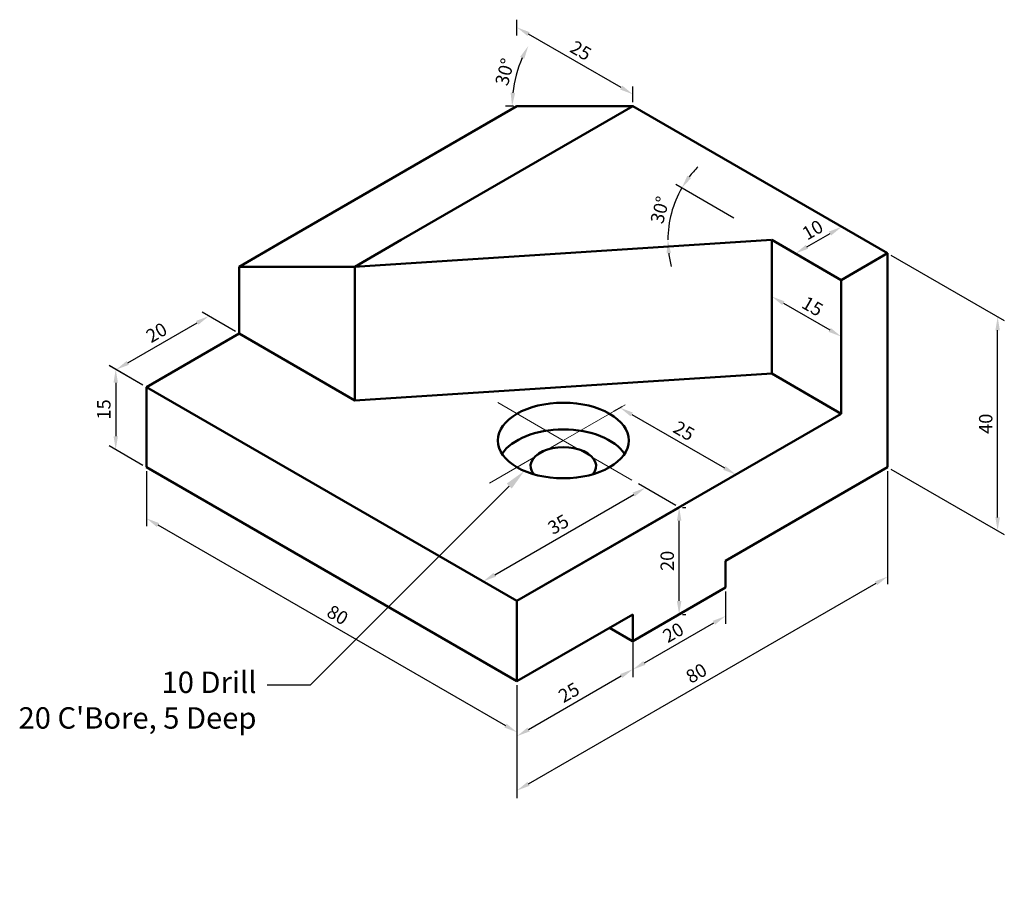
# Model space of a CAD drawing. Units: millimetres. Extents: x 2441 to 2625, y 4324 to 4485.
import ezdxf
from ezdxf import colors
from ezdxf.entities.mleader import LeaderData, LeaderLine
from ezdxf.math import Vec2, Vec3

# ---------------------------------------------------------------- set-up
doc = ezdxf.new("R2010")
doc.units = ezdxf.units.MM
doc.linetypes.add('CENTER', pattern=[50.8, 31.75, -6.35, 6.35, -6.35])
for name, color, linetype, lineweight in [('M-CNTR', 4, 'CENTER', 18), ('M-DIMS', 2, 'Continuous', 25), ('M-OUTL', 7, 'Continuous', 50), ('M-TEXT', 7, 'Continuous', 25)]:
    doc.layers.add(name, color=color, linetype=linetype, lineweight=lineweight)
doc.styles.get("Standard").update_dxf_attribs({"font": 'arial.ttf'})
doc.dimstyles.new('ISO-25', dxfattribs={"dimtxt": 2.5, "dimasz": 2.5, "dimexe": 1.25, "dimexo": 0.625, "dimtad": 1, "dimtxsty": 'Standard', "dimcen": 2.5, "dimadec": 0, "dimazin": 0, "dimtfac": 1, "dimtmove": 0, "dimatfit": 3, "dimfxl": 1, "dimarcsym": 0})

# ---------------------------------------------------------------- blocks, each defined once
blk = doc.blocks.new('*D1')
at = {"layer": 'Defpoints', "color": 0, "transparency": 16777216}
for p in [(2594.92, 4446.26), (2603.5, 4441.3), (2594.84, 4436.3)]:
    blk.add_point(p, dxfattribs=at)
at = {"layer": 'M-DIMS', "color": 0, "lineweight": -2, "transparency": 16777216}
for p, q in [((2602.88, 4441.66), (2593.67, 4446.98)), ((2588.42, 4442.51), (2592.75, 4445.01)), ((2594.22, 4436.66), (2585.01, 4441.98))]:
    blk.add_line(p, q, dxfattribs=at)
at = {"layer": 'M-DIMS', "color": 0, "transparency": 16777216}
for points in [[(2592.54, 4445.37), (2592.96, 4444.65), (2594.92, 4446.26)], [(2588.21, 4442.87), (2588.63, 4442.15), (2586.26, 4441.26)]]:
    blk.add_solid(points, dxfattribs=at)
at = {"layer": 'M-DIMS', "color": 0, "transparency": 16777216, "insert": (2589.64, 4445.41), "char_height": 2.5, "attachment_point": 5, "rotation": 30}
blk.add_mtext('10', dxfattribs=at)
blk = doc.blocks.new('*D2')
at = {"layer": 'Defpoints', "color": 0, "transparency": 16777216}
for p in [(2534.22, 4483.54), (2534.22, 4481.3), (2555.87, 4468.8)]:
    blk.add_point(p, dxfattribs=at)
at = {"layer": 'M-DIMS', "color": 0, "lineweight": -2, "transparency": 16777216}
for p, q in [((2534.22, 4482.03), (2534.22, 4484.98)), ((2553.7, 4472.29), (2536.38, 4482.29)), ((2555.87, 4469.53), (2555.87, 4472.48))]:
    blk.add_line(p, q, dxfattribs=at)
at = {"layer": 'M-DIMS', "color": 0, "transparency": 16777216}
for points in [[(2536.59, 4482.65), (2536.18, 4481.93), (2534.22, 4483.54)], [(2553.91, 4472.65), (2553.5, 4471.93), (2555.87, 4471.04)]]:
    blk.add_solid(points, dxfattribs=at)
at = {"layer": 'M-DIMS', "color": 0, "transparency": 16777216, "insert": (2545.99, 4478.93), "char_height": 2.5, "attachment_point": 5, "rotation": 330}
blk.add_mtext('25', dxfattribs=at)
blk = doc.blocks.new('*D3')
at = {"layer": 'Defpoints', "color": 0, "transparency": 16777216}
for p in [(2534.22, 4481.3), (2534.67, 4476.52), (2534.22, 4468.8), (2555.87, 4468.8), (2555.87, 4468.8)]:
    blk.add_point(p, dxfattribs=at)
at = {"layer": 'M-DIMS', "color": 0, "lineweight": -2, "transparency": 16777216}
blk.add_line((2533.59, 4468.8), (2532.06, 4468.8), dxfattribs=at)
blk.add_arc((2555.87, 4468.8), 22.56, 156.3532, 173.6468, dxfattribs=at)
at = {"layer": 'M-DIMS', "color": 0, "transparency": 16777216}
for points in [[(2534.83, 4478.04), (2535.58, 4477.66), (2536.33, 4480.08)], [(2533.87, 4471.28), (2533.03, 4471.32), (2533.31, 4468.8)]]:
    blk.add_solid(points, dxfattribs=at)
at = {"layer": 'M-DIMS', "color": 0, "transparency": 16777216, "insert": (2532.24, 4475.13), "char_height": 2.5, "attachment_point": 5, "rotation": 75}
blk.add_mtext('30°', dxfattribs=at)
blk = doc.blocks.new('*D4')
at = {"layer": 'Defpoints', "color": 0, "transparency": 16777216}
for p in [(2603.5, 4441.3), (2624.06, 4429.43), (2603.5, 4401.3)]:
    blk.add_point(p, dxfattribs=at)
at = {"layer": 'M-DIMS', "color": 0, "lineweight": -2, "transparency": 16777216}
for p, q in [((2604.13, 4440.94), (2625.31, 4428.71)), ((2624.06, 4391.93), (2624.06, 4426.93)), ((2604.13, 4400.94), (2625.31, 4388.71))]:
    blk.add_line(p, q, dxfattribs=at)
at = {"layer": 'M-DIMS', "color": 0, "transparency": 16777216}
for points in [[(2623.65, 4426.93), (2624.48, 4426.93), (2624.06, 4429.43)], [(2623.65, 4391.93), (2624.48, 4391.93), (2624.06, 4389.43)]]:
    blk.add_solid(points, dxfattribs=at)
at = {"layer": 'M-DIMS', "color": 0, "transparency": 16777216, "insert": (2622.16, 4409.43), "char_height": 2.5, "attachment_point": 5, "rotation": 90}
blk.add_mtext('40', dxfattribs=at)
blk = doc.blocks.new('*D5')
at = {"layer": 'Defpoints', "color": 0, "transparency": 16777216}
for p in [(2476.61, 4429.56), (2482.26, 4426.3), (2464.94, 4416.3)]:
    blk.add_point(p, dxfattribs=at)
at = {"layer": 'M-DIMS', "color": 0, "lineweight": -2, "transparency": 16777216}
for p, q in [((2481.63, 4426.66), (2475.36, 4430.28)), ((2461.46, 4420.81), (2474.45, 4428.31)), ((2464.31, 4416.66), (2458.04, 4420.28))]:
    blk.add_line(p, q, dxfattribs=at)
at = {"layer": 'M-DIMS', "color": 0, "transparency": 16777216}
for points in [[(2474.24, 4428.67), (2474.66, 4427.95), (2476.61, 4429.56)], [(2461.25, 4421.17), (2461.67, 4420.45), (2459.29, 4419.56)]]:
    blk.add_solid(points, dxfattribs=at)
at = {"layer": 'M-DIMS', "color": 0, "transparency": 16777216, "insert": (2467, 4426.21), "char_height": 2.5, "attachment_point": 5, "rotation": 30}
blk.add_mtext('20', dxfattribs=at)
blk = doc.blocks.new('*D6')
at = {"layer": 'Defpoints', "color": 0, "transparency": 16777216}
for p in [(2464.94, 4416.3), (2459.21, 4404.61), (2464.94, 4401.3)]:
    blk.add_point(p, dxfattribs=at)
at = {"layer": 'M-DIMS', "color": 0, "lineweight": -2, "transparency": 16777216}
for p, q in [((2464.31, 4416.66), (2457.96, 4420.33)), ((2459.21, 4417.11), (2459.21, 4407.11)), ((2464.31, 4401.66), (2457.96, 4405.33))]:
    blk.add_line(p, q, dxfattribs=at)
at = {"layer": 'M-DIMS', "color": 0, "transparency": 16777216}
for points in [[(2458.8, 4417.11), (2459.63, 4417.11), (2459.21, 4419.61)], [(2458.8, 4407.11), (2459.63, 4407.11), (2459.21, 4404.61)]]:
    blk.add_solid(points, dxfattribs=at)
at = {"layer": 'M-DIMS', "color": 0, "transparency": 16777216, "insert": (2457.31, 4412.11), "char_height": 2.5, "attachment_point": 5, "rotation": 90}
blk.add_mtext('15', dxfattribs=at)
blk = doc.blocks.new('*D7')
at = {"layer": 'Defpoints', "color": 0, "transparency": 16777216}
for p in [(2464.94, 4401.3), (2534.22, 4361.3), (2534.22, 4351.76)]:
    blk.add_point(p, dxfattribs=at)
at = {"layer": 'M-DIMS', "color": 0, "lineweight": -2, "transparency": 16777216}
for p, q in [((2464.94, 4400.58), (2464.94, 4390.32)), ((2467.1, 4390.51), (2532.05, 4353.01)), ((2534.22, 4360.58), (2534.22, 4350.32))]:
    blk.add_line(p, q, dxfattribs=at)
at = {"layer": 'M-DIMS', "color": 0, "transparency": 16777216}
for points in [[(2467.31, 4390.87), (2466.89, 4390.15), (2464.94, 4391.76)], [(2532.26, 4353.37), (2531.85, 4352.65), (2534.22, 4351.76)]]:
    blk.add_solid(points, dxfattribs=at)
at = {"layer": 'M-DIMS', "color": 0, "transparency": 16777216, "insert": (2500.53, 4373.41), "char_height": 2.5, "attachment_point": 5, "rotation": 330}
blk.add_mtext('80', dxfattribs=at)
blk = doc.blocks.new('*D8')
at = {"layer": 'Defpoints', "color": 0, "transparency": 16777216}
for p in [(2555.87, 4373.8), (2555.87, 4363.53), (2534.22, 4361.3)]:
    blk.add_point(p, dxfattribs=at)
at = {"layer": 'M-DIMS', "color": 0, "lineweight": -2, "transparency": 16777216}
for p, q in [((2555.87, 4373.08), (2555.87, 4362.08)), ((2536.38, 4352.28), (2553.7, 4362.28)), ((2534.22, 4360.58), (2534.22, 4349.58))]:
    blk.add_line(p, q, dxfattribs=at)
at = {"layer": 'M-DIMS', "color": 0, "transparency": 16777216}
for points in [[(2553.5, 4362.64), (2553.91, 4361.91), (2555.87, 4363.53)], [(2536.18, 4352.64), (2536.59, 4351.91), (2534.22, 4351.03)]]:
    blk.add_solid(points, dxfattribs=at)
at = {"layer": 'M-DIMS', "color": 0, "transparency": 16777216, "insert": (2544.09, 4358.92), "char_height": 2.5, "attachment_point": 5, "rotation": 30}
blk.add_mtext('25', dxfattribs=at)
blk = doc.blocks.new('*D9')
at = {"layer": 'Defpoints', "color": 0, "transparency": 16777216}
for p in [(2573.19, 4378.8), (2573.19, 4373.48), (2555.87, 4368.8)]:
    blk.add_point(p, dxfattribs=at)
at = {"layer": 'M-DIMS', "color": 0, "lineweight": -2, "transparency": 16777216}
for p, q in [((2573.19, 4378.08), (2573.19, 4372.04)), ((2558.03, 4364.73), (2571.02, 4372.23)), ((2555.87, 4368.08), (2555.87, 4362.04))]:
    blk.add_line(p, q, dxfattribs=at)
at = {"layer": 'M-DIMS', "color": 0, "transparency": 16777216}
for points in [[(2570.82, 4372.59), (2571.23, 4371.87), (2573.19, 4373.48)], [(2557.83, 4365.09), (2558.24, 4364.37), (2555.87, 4363.48)]]:
    blk.add_solid(points, dxfattribs=at)
at = {"layer": 'M-DIMS', "color": 0, "transparency": 16777216, "insert": (2563.58, 4370.13), "char_height": 2.5, "attachment_point": 5, "rotation": 30}
blk.add_mtext('20', dxfattribs=at)
blk = doc.blocks.new('*D10')
at = {"layer": 'Defpoints', "color": 0, "transparency": 16777216}
for p in [(2603.5, 4401.3), (2603.5, 4380.87), (2534.22, 4361.3)]:
    blk.add_point(p, dxfattribs=at)
at = {"layer": 'M-DIMS', "color": 0, "lineweight": -2, "transparency": 16777216}
for p, q in [((2603.5, 4400.58), (2603.5, 4379.43)), ((2536.38, 4342.12), (2601.34, 4379.62)), ((2534.22, 4360.58), (2534.22, 4339.43))]:
    blk.add_line(p, q, dxfattribs=at)
at = {"layer": 'M-DIMS', "color": 0, "transparency": 16777216}
for points in [[(2601.13, 4379.98), (2601.54, 4379.26), (2603.5, 4380.87)], [(2536.18, 4342.48), (2536.59, 4341.76), (2534.22, 4340.87)]]:
    blk.add_solid(points, dxfattribs=at)
at = {"layer": 'M-DIMS', "color": 0, "transparency": 16777216, "insert": (2567.91, 4362.52), "char_height": 2.5, "attachment_point": 5, "rotation": 30}
blk.add_mtext('80', dxfattribs=at)
blk = doc.blocks.new('*D11')
at = {"layer": 'Defpoints', "color": 0, "transparency": 16777216}
for p in [(2564.53, 4393.8), (2564.53, 4393.8), (2564.53, 4373.8)]:
    blk.add_point(p, dxfattribs=at)
at = {"layer": 'M-DIMS', "color": 0, "lineweight": -2, "transparency": 16777216}
for p, q in [((2565.15, 4393.8), (2565.78, 4393.8)), ((2564.53, 4376.3), (2564.53, 4391.3)), ((2565.15, 4373.8), (2565.78, 4373.8))]:
    blk.add_line(p, q, dxfattribs=at)
at = {"layer": 'M-DIMS', "color": 0, "transparency": 16777216}
for points in [[(2564.11, 4391.3), (2564.95, 4391.3), (2564.53, 4393.8)], [(2564.11, 4376.3), (2564.95, 4376.3), (2564.53, 4373.8)]]:
    blk.add_solid(points, dxfattribs=at)
at = {"layer": 'M-DIMS', "color": 0, "transparency": 16777216, "insert": (2562.63, 4383.8), "char_height": 2.5, "attachment_point": 5, "rotation": 90}
blk.add_mtext('20', dxfattribs=at)
blk = doc.blocks.new('*D12')
at = {"layer": 'Defpoints', "color": 0, "transparency": 16777216}
for p in [(2558.2, 4397.46), (2564.53, 4393.8), (2534.22, 4376.3)]:
    blk.add_point(p, dxfattribs=at)
at = {"layer": 'M-DIMS', "color": 0, "lineweight": -2, "transparency": 16777216}
for p, q in [((2563.9, 4394.16), (2556.95, 4398.18)), ((2530.06, 4381.21), (2556.04, 4396.21)), ((2533.59, 4376.66), (2526.64, 4380.68))]:
    blk.add_line(p, q, dxfattribs=at)
at = {"layer": 'M-DIMS', "color": 0, "transparency": 16777216}
for points in [[(2555.83, 4396.57), (2556.25, 4395.84), (2558.2, 4397.46)], [(2529.85, 4381.57), (2530.27, 4380.84), (2527.89, 4379.96)]]:
    blk.add_solid(points, dxfattribs=at)
at = {"layer": 'M-DIMS', "color": 0, "transparency": 16777216, "insert": (2542.1, 4390.35), "char_height": 2.5, "attachment_point": 5, "rotation": 30}
blk.add_mtext('35', dxfattribs=at)
blk = doc.blocks.new('*D13')
at = {"layer": 'Defpoints', "color": 0, "transparency": 16777216}
for p in [(2554.46, 4412.99), (2575.14, 4399.93), (2576.11, 4400.49)]:
    blk.add_point(p, dxfattribs=at)
at = {"layer": 'M-DIMS', "color": 0, "lineweight": -2, "transparency": 16777216}
for p, q in [((2553.83, 4412.63), (2552.24, 4411.71)), ((2555.66, 4411.18), (2572.98, 4401.18)), ((2575.48, 4400.13), (2573.89, 4399.21))]:
    blk.add_line(p, q, dxfattribs=at)
at = {"layer": 'M-DIMS', "color": 0, "transparency": 16777216}
for points in [[(2555.87, 4411.54), (2555.45, 4410.82), (2553.49, 4412.43)], [(2573.19, 4401.54), (2572.77, 4400.82), (2575.14, 4399.93)]]:
    blk.add_solid(points, dxfattribs=at)
at = {"layer": 'M-DIMS', "color": 0, "transparency": 16777216, "insert": (2565.27, 4407.83), "char_height": 2.5, "attachment_point": 5, "rotation": 330}
blk.add_mtext('25', dxfattribs=at)
blk = doc.blocks.new('*D14')
at = {"layer": 'Defpoints', "color": 0, "transparency": 16777216}
for p in [(2581.85, 4443.8), (2594.84, 4436.3), (2594.84, 4425.73)]:
    blk.add_point(p, dxfattribs=at)
at = {"layer": 'M-DIMS', "color": 0, "lineweight": -2, "transparency": 16777216}
for p, q in [((2581.85, 4443.08), (2581.85, 4431.78)), ((2594.84, 4435.58), (2594.84, 4424.28)), ((2584.02, 4431.98), (2592.68, 4426.98))]:
    blk.add_line(p, q, dxfattribs=at)
at = {"layer": 'M-DIMS', "color": 0, "transparency": 16777216}
for points in [[(2584.22, 4432.34), (2583.81, 4431.62), (2581.85, 4433.23)], [(2592.88, 4427.34), (2592.47, 4426.62), (2594.84, 4425.73)]]:
    blk.add_solid(points, dxfattribs=at)
at = {"layer": 'M-DIMS', "color": 0, "transparency": 16777216, "insert": (2589.3, 4431.12), "char_height": 2.5, "attachment_point": 5, "rotation": 330}
blk.add_mtext('15', dxfattribs=at)
blk = doc.blocks.new('*D15')
at = {"layer": 'Defpoints', "color": 0, "transparency": 16777216}
for p in [(2563.6, 4450.45), (2575.32, 4447.57), (2512.57, 4443.8), (2581.85, 4443.8), (2581.85, 4443.8)]:
    blk.add_point(p, dxfattribs=at)
at = {"layer": 'M-DIMS', "color": 0, "lineweight": -2, "transparency": 16777216}
blk.add_line((2574.78, 4447.88), (2563.94, 4454.14), dxfattribs=at)
for start, end in [(135.243, 142.6215), (150, 180), (187.3785, 194.757)]:
    blk.add_arc((2581.85, 4443.8), 19.43, start, end, dxfattribs=at)
at = {"layer": 'M-DIMS', "color": 0, "transparency": 16777216}
for points in [[(2566.76, 4455.37), (2566.07, 4455.83), (2565.03, 4453.52)], [(2562.17, 4441.28), (2563, 4441.34), (2562.42, 4443.8)]]:
    blk.add_solid(points, dxfattribs=at)
at = {"layer": 'M-DIMS', "color": 0, "transparency": 16777216, "insert": (2561.25, 4449.32), "char_height": 2.5, "attachment_point": 5, "rotation": 75}
blk.add_mtext('30°', dxfattribs=at)

msp = doc.modelspace()

# ---------------------------------------------------------------- linework, layer by layer
at = {"layer": 'M-CNTR'}
for p, q in [((2542.879, 4406.303), (2530.61, 4413.387)), ((2542.879, 4406.303), (2554.459, 4412.989)), ((2542.879, 4406.303), (2529.107, 4398.352)), ((2555.683, 4398.911), (2542.879, 4406.303))]:
    msp.add_line(p, q, dxfattribs=at)
at = {"layer": 'M-OUTL'}
for p, q in [((2534.219, 4468.803), (2490.173, 4443.373)), ((2555.869, 4468.803), (2512.568, 4443.803)), ((2555.869, 4468.803), (2534.219, 4468.803)), ((2603.501, 4441.303), (2555.869, 4468.803)), ((2490.173, 4443.373), (2482.257, 4438.803)), ((2503.868, 4438.803), (2581.81, 4443.803)), ((2512.568, 4443.803), (2503.908, 4438.803)), ((2594.841, 4436.303), (2581.85, 4443.803)), ((2594.841, 4436.303), (2581.85, 4443.803)), ((2581.85, 4443.803), (2581.85, 4418.803)), ((2603.501, 4441.303), (2594.841, 4436.303)), ((2603.501, 4401.303), (2603.501, 4441.303)), ((2482.257, 4426.303), (2482.257, 4438.803)), ((2482.257, 4438.803), (2503.908, 4438.803)), ((2503.908, 4413.803), (2503.908, 4438.803)), ((2594.841, 4436.303), (2594.841, 4411.303)), ((2464.937, 4416.303), (2482.257, 4426.303)), ((2482.257, 4426.303), (2495.248, 4418.803)), ((2482.257, 4426.303), (2503.908, 4413.803)), ((2503.908, 4413.803), (2503.908, 4422.919)), ((2581.85, 4418.803), (2503.908, 4413.803)), ((2594.841, 4411.303), (2581.85, 4418.803)), ((2534.219, 4376.303), (2464.937, 4416.303)), ((2464.937, 4416.303), (2464.937, 4401.303)), ((2534.219, 4376.303), (2594.841, 4411.303)), ((2464.937, 4401.303), (2534.219, 4361.303)), ((2573.19, 4383.803), (2603.501, 4401.303)), ((2534.219, 4376.303), (2564.53, 4393.803)), ((2573.19, 4383.803), (2573.19, 4378.803)), ((2555.869, 4368.803), (2573.19, 4378.803)), ((2534.219, 4361.303), (2534.219, 4376.303)), ((2534.219, 4361.303), (2555.869, 4373.803)), ((2534.219, 4361.303), (2555.869, 4373.803)), ((2555.869, 4373.803), (2555.869, 4368.803)), ((2555.869, 4373.803), (2555.869, 4368.803)), ((2555.829, 4368.803), (2551.499, 4371.303))]:
    msp.add_line(p, q, dxfattribs=at)
msp.add_ellipse((2542.879, 4406.303), major_axis=(-12.247, 0), ratio=0.5773503, dxfattribs=at)
for centre, major_axis, start_param, end_param in [((2542.879, 4401.303), (-12.247, 0), 3.5029598, 5.9218182), ((2542.879, 4401.519), (-6.124, 0), 2.6951189, 6.7296591)]:
    msp.add_ellipse(centre, major_axis=major_axis, ratio=0.5773503, start_param=start_param, end_param=end_param, dxfattribs=at)

# ---------------------------------------------------------------- dimensions: what is measured, and where the dimension line sits
at = {"layer": 'M-DIMS'}
for p1, p2, distance, picture, middle in [((2555.869, 4468.803), (2534.219, 4481.303), -1.934, '*D2', (2545.995, 4478.933)), ((2594.841, 4436.303), (2603.501, 4441.303), 8.583, '*D1', (2589.637, 4445.406)), ((2581.85, 4443.803), (2594.841, 4436.303), -9.158, '*D14', (2589.296, 4431.125)), ((2464.937, 4416.303), (2482.257, 4426.303), 5.643, '*D5', (2467.003, 4426.208)), ((2464.937, 4416.303), (2464.937, 4401.303), -5.725, '*D6', (2457.311, 4412.108)), ((2554.459, 4412.989), (2576.11, 4400.489), -0.966, '*D13', (2565.269, 4407.828)), ((2464.937, 4401.303), (2534.219, 4361.303), -8.266, '*D7', (2500.528, 4373.405)), ((2534.219, 4361.303), (2603.501, 4401.303), -17.697, '*D10', (2567.909, 4362.516)), ((2534.219, 4376.303), (2564.53, 4393.803), 6.325, '*D12', (2542.098, 4390.353)), ((2564.53, 4373.803), (2564.53, 4393.803), 0, '*D11', (2562.628, 4383.803)), ((2555.869, 4368.803), (2573.19, 4378.803), -4.609, '*D9', (2563.579, 4370.128)), ((2534.219, 4361.303), (2555.869, 4373.803), -8.901, '*D8', (2544.093, 4358.922))]:
    dim = msp.add_aligned_dim(p1=p1, p2=p2, distance=distance, dimstyle='ISO-25', override={"dimclrd": 0, "dimclre": 0, "dimclrt": 0}, dxfattribs=at)
    dim.commit()
    dim.dimension.update_dxf_attribs({"geometry": picture, "text_midpoint": middle})
for base, line1, line2, picture, middle in [((2534.672, 4476.519), ((2555.869, 4468.803), (2534.219, 4468.803)), ((2555.869, 4468.803), (2534.219, 4481.303)), '*D3', (2532.243, 4475.134)), ((2563.595, 4450.448), ((2581.85, 4443.803), (2575.323, 4447.572)), ((2581.85, 4443.803), (2512.568, 4443.803)), '*D15', (2561.248, 4449.324))]:
    dim = msp.add_angular_dim_2l(base=base, line1=line1, line2=line2, dimstyle='ISO-25', override={"dimclrd": 0, "dimclre": 0, "dimclrt": 0}, dxfattribs=at)
    dim.commit()
    dim.dimension.update_dxf_attribs({"geometry": picture, "text_midpoint": middle})
dim = msp.add_linear_dim(base=(2624.062, 4429.432), p1=(2603.501, 4401.303), p2=(2603.501, 4441.303), angle=90, dimstyle='ISO-25', override={"dimclrd": 0, "dimclre": 0, "dimclrt": 0}, dxfattribs=at)
dim.commit()
dim.dimension.update_dxf_attribs({"geometry": '*D4', "text_midpoint": (2622.16, 4409.432)})

# ---------------------------------------------------------------- leaders
at = {"layer": 'M-TEXT'}
ml = msp.add_multileader_mtext('Standard', dxfattribs=at)
ml.set_content("10 Drill\\P20 C'Bore, 5 Deep", color=256)
ml.set_leader_properties()
ml.build(insert=Vec2(0, 0))
ctx = ml.context
ctx.base_point, ctx.plane_origin = Vec3(2438.117, 4360.547), Vec3(2535.599, 4400.617)
ctx.text_align_type = 2
notes = []
notes.append((ctx, [(0, (1, 1, 0), (2495.528, 4360.547), (-1, 0), 8, [(0, [(2535.599, 4400.617)], 0, [])])]))
ctx.mtext.insert, ctx.mtext.alignment, ctx.mtext.flow_direction = Vec3(2485.528, 4363.102), 3, 5
for ctx, leaders in notes:
    for number, flags, end, landing, length, lines in leaders:
        leader = LeaderData()
        leader.index, (leader.has_last_leader_line, leader.has_dogleg_vector, leader.attachment_direction) = number, flags
        leader.last_leader_point, leader.dogleg_vector, leader.dogleg_length = Vec3(end), Vec3(landing), length
        for number, points, colour, breaks in lines:
            line = LeaderLine()
            line.index, line.vertices, line.color, line.breaks = number, Vec3.list(points), colors.encode_raw_color(colour), breaks
            leader.lines.append(line)
        ctx.leaders.append(leader)

doc.saveas('drawing.dxf')
